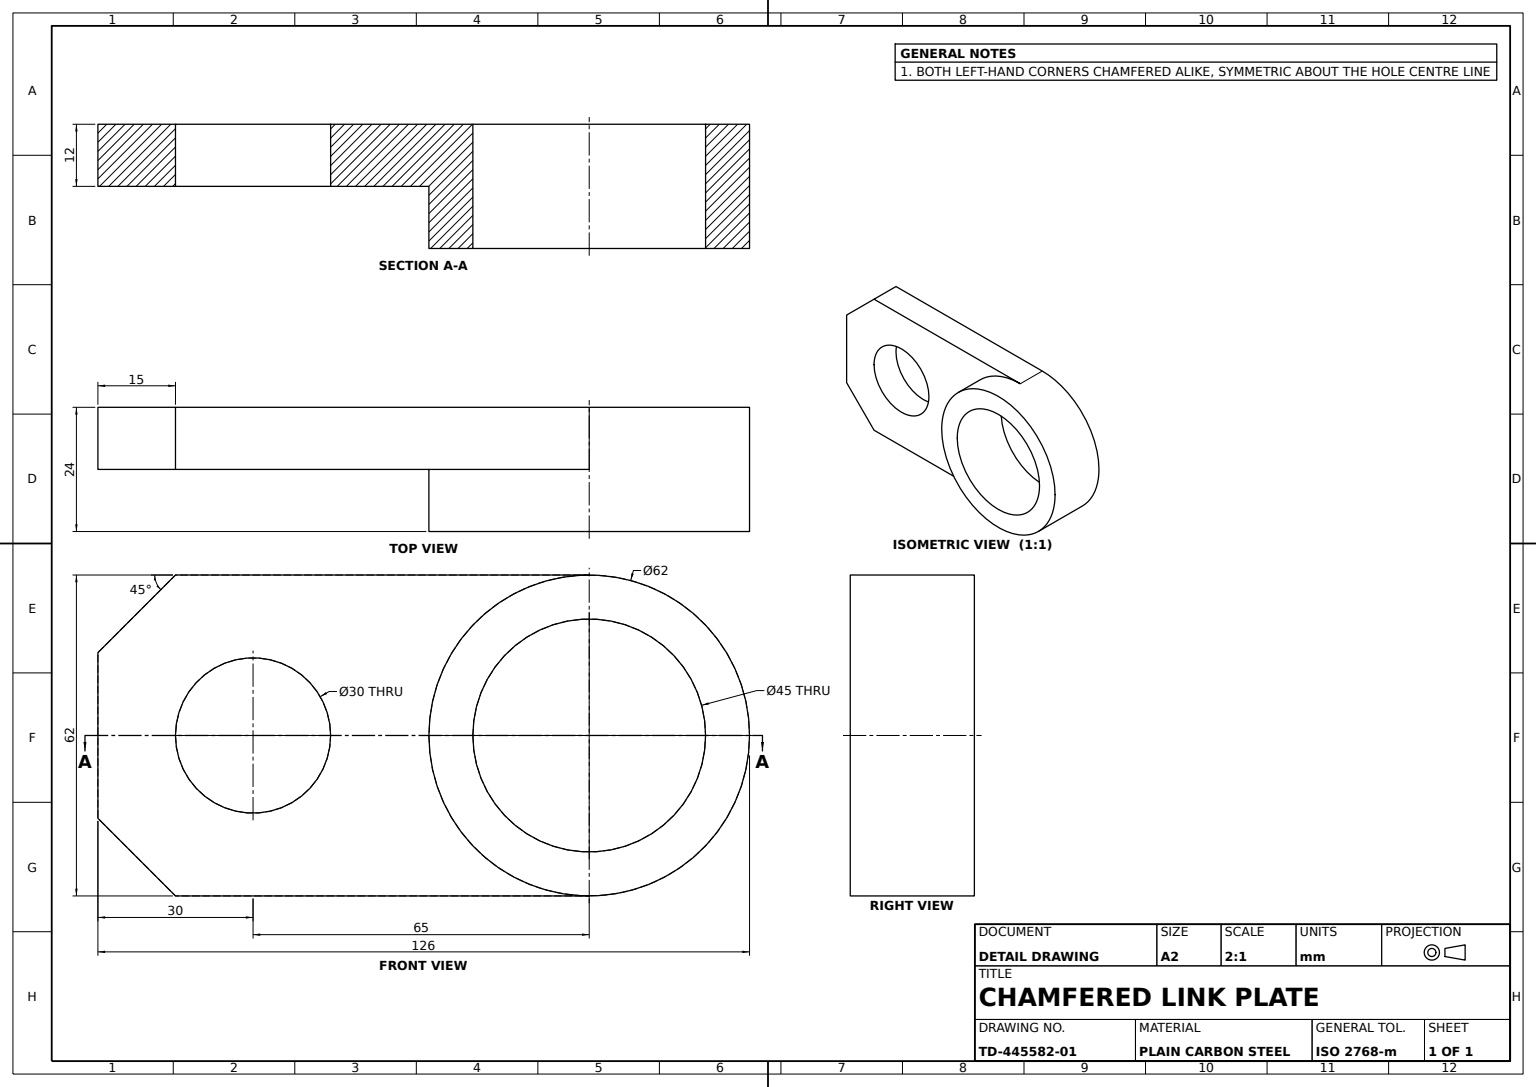
SolidWorks part; units mm, degrees
material "Plain Carbon Steel"
ref_plane "Front Plane" through (0, 0, 0) normal (0, 0, 1) x (1, 0, 0)
ref_plane "Top Plane" through (0, 0, 0) normal (0, 1, 0) x (1, 0, 0)
ref_plane "Right Plane" through (0, 0, 0) normal (1, 0, 0) x (0, 0, -1)
sketch "Base Plate Sketch" plane through (0, 0, 0) normal (0, 0, 1) x (1, 0, 0)
  line L2 (65, -31) -> (-15, -31)
  line L3 (65, 31) -> (-15, 31)
  line L4 (-30, 0) -> (-30, 16)
  line L5 (-30, 16) -> (-30, -16)
  line L7 (-15, 31) -> (-30, 16)
  line L9 (-15, -31) -> (-30, -16)
  arc A0 (65, -31) -> (65, 31) centre (65, 0) ccw
  dimension "D1" = 62
  dimension "D2" = 15
  dimension "D3" = 15
  dimension "D4" = 32
  dimension "D5" = 65
  dimension "D6" = 80
  dimension "D7" = 30
extrude "Base Plate" add sketch "Base Plate Sketch" along normal blind 12 contours L2 A0 L3 L7 L4 L5 L9
sketch "Boss Sketch Ø62" plane through (0, 0, 12) normal (0, 0, 1) x (1, 0, 0)
  circle A0 centre (65, 0) radius 31
  dimension "D1" = 62
  dimension "D2" = 62
extrude "Boss Ø62" add sketch "Boss Sketch Ø62" along normal blind 12
sketch "Bore Sketch Ø45" plane through (0, 0, 24) normal (0, 0, 1) x (1, 0, 0)
  circle A0 centre (65, 0) radius 22.5
  dimension "D1" = 45
  dimension "D2" = 45
extrude "Bore Ø45" cut sketch "Bore Sketch Ø45" against normal blind 25
sketch "Hole Sketch Ø30" plane through (0, 0, 12) normal (0, 0, 1) x (1, 0, 0)
  circle A0 centre (0, 0) radius 15
  dimension "D1" = 30
  dimension "D2" = 30
extrude "Hole Ø30" cut sketch "Hole Sketch Ø30" against normal blind 25
